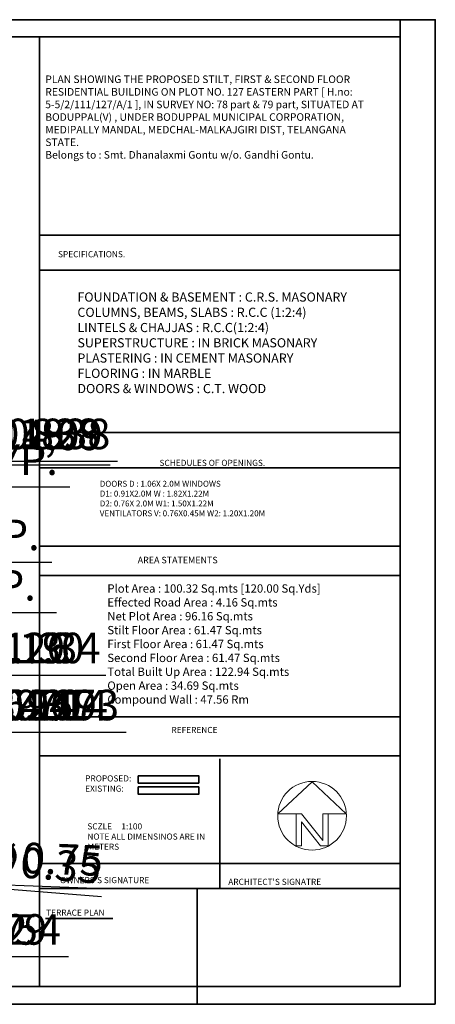
# Model space of a CAD drawing. Units: metres. Extents: x 782 to 1487, y 1262 to 7446.
# Tile 25 of 25: x 850 to 884, y 1262 to 1343. Entities that reach past the tile are written whole.
import ezdxf

# ---------------------------------------------------------------- set-up
doc = ezdxf.new("R2010")
doc.units = ezdxf.units.M
for name, color, linetype, lineweight in [('A-ANNO-DIMS', 2, 'Continuous', 18), ('A-ANNO-SYMB', 7, 'Continuous', 18), ('A-ANNO-TTLB', 7, 'Continuous', 35)]:
    doc.layers.add(name, color=color, linetype=linetype, lineweight=lineweight)
doc.styles.get("Standard").update_dxf_attribs({"font": 'arial.ttf'})
doc.dimstyles.new('ISO-25', dxfattribs={"dimtxt": 2.5, "dimasz": 2.5, "dimexe": 1.25, "dimexo": 0.625, "dimtad": 1, "dimtxsty": 'Standard', "dimcen": 2.5, "dimadec": 0, "dimazin": 0, "dimtfac": 1, "dimtmove": 0, "dimatfit": 3, "dimfxl": 1, "dimarcsym": 0})

# ---------------------------------------------------------------- blocks, each defined once
blk = doc.blocks.new('*D9')
at = {"layer": 'A-ANNO-DIMS', "color": 0, "lineweight": -2, "transparency": 16777216}
for p, q in [((840.095, 1306.46), (840.095, 1307.78)), ((844.185, 1306.46), (844.185, 1307.78)), ((837.595, 1306.53), (835.095, 1306.53)), ((840.095, 1306.53), (844.185, 1306.53)), ((846.685, 1306.53), (857.034, 1306.53))]:
    blk.add_line(p, q, dxfattribs=at)
at = {"layer": 'A-ANNO-DIMS', "color": 0, "transparency": 16777216}
for points in [[(837.595, 1306.947), (837.595, 1306.114), (840.095, 1306.53)], [(846.685, 1306.947), (846.685, 1306.114), (844.185, 1306.53)]]:
    blk.add_solid(points, dxfattribs=at)
at = {"layer": 'Defpoints', "color": 0, "transparency": 16777216}
for p in [(844.185, 1306.53), (840.095, 1305.835), (844.185, 1305.835)]:
    blk.add_point(p, dxfattribs=at)
at = {"layer": 'A-ANNO-DIMS', "color": 0, "transparency": 16777216, "insert": (853.11, 1308.658), "char_height": 2.5, "attachment_point": 5}
blk.add_mtext('4,09', dxfattribs=at)
blk = doc.blocks.new('North Arrow')
for p, q in [((0, 0), (-12.86, -11.999)), ((0, 0), (12.782, -11.999)), ((-12.86, -11.999), (-6, -11.999)), ((-6, -11.999), (-6, -23.999)), ((-6, -11.999), (-4, -11.999)), ((-4, -11.999), (4, -21.999)), ((4, -11.999), (4, -21.999)), ((6, -11.999), (4, -11.999)), ((12.782, -11.999), (6, -11.999)), ((6, -11.999), (6, -23.999)), ((3.195, -23.996), (-4, -15.002)), ((-4, -15.002), (-4, -23.999)), ((-6, -23.999), (-4, -23.999)), ((6, -23.999), (3.195, -23.999))]:
    blk.add_line(p, q)
blk.add_circle((-0.013, -12.745), 12.885)
blk = doc.blocks.new('*D21')
at = {"layer": 'A-ANNO-DIMS', "color": 0, "lineweight": -2, "transparency": 16777216}
for p, q in [((827.576, 1298.565), (825.076, 1298.565)), ((830.076, 1298.565), (830.923, 1298.565)), ((833.423, 1298.565), (852.255, 1298.565)), ((830.076, 1298.073), (830.076, 1297.315)), ((830.923, 1298.073), (830.923, 1297.315))]:
    blk.add_line(p, q, dxfattribs=at)
at = {"layer": 'A-ANNO-DIMS', "color": 0, "transparency": 16777216}
for points in [[(827.576, 1298.981), (827.576, 1298.148), (830.076, 1298.565)], [(833.423, 1298.981), (833.423, 1298.148), (830.923, 1298.565)]]:
    blk.add_solid(points, dxfattribs=at)
at = {"layer": 'Defpoints', "color": 0, "transparency": 16777216}
for p in [(830.076, 1298.698), (830.923, 1298.698), (830.923, 1298.565)]:
    blk.add_point(p, dxfattribs=at)
at = {"layer": 'A-ANNO-DIMS', "color": 0, "transparency": 16777216, "insert": (844.089, 1300.466), "char_height": 2.5, "attachment_point": 5}
blk.add_mtext('0.85 TYP.', dxfattribs=at)
blk = doc.blocks.new('*D24')
at = {"layer": 'A-ANNO-DIMS', "color": 0, "lineweight": -2, "transparency": 16777216}
for p, q in [((811.209, 1294.423), (808.709, 1294.423)), ((813.709, 1294.423), (814.559, 1294.423)), ((817.059, 1294.423), (852.649, 1294.423)), ((813.709, 1293.926), (813.709, 1293.173)), ((814.559, 1293.926), (814.559, 1293.173))]:
    blk.add_line(p, q, dxfattribs=at)
at = {"layer": 'A-ANNO-DIMS', "color": 0, "transparency": 16777216}
for points in [[(811.209, 1294.84), (811.209, 1294.006), (813.709, 1294.423)], [(817.059, 1294.84), (817.059, 1294.006), (814.559, 1294.423)]]:
    blk.add_solid(points, dxfattribs=at)
at = {"layer": 'Defpoints', "color": 0, "transparency": 16777216}
for p in [(813.709, 1294.551), (814.559, 1294.551), (814.559, 1294.423)]:
    blk.add_point(p, dxfattribs=at)
at = {"layer": 'A-ANNO-DIMS', "color": 0, "transparency": 16777216, "insert": (836.104, 1296.342), "char_height": 2.5, "attachment_point": 5}
blk.add_mtext('DOOR D2 0.85 TYP.', dxfattribs=at)
blk = doc.blocks.new('*D29')
at = {"layer": 'A-ANNO-DIMS', "color": 0, "lineweight": -2, "transparency": 16777216}
for p, q in [((829.683, 1304.73), (827.183, 1304.73)), ((832.183, 1304.73), (832.413, 1304.73)), ((832.183, 1304.242), (832.183, 1303.48)), ((832.413, 1304.242), (832.413, 1303.48)), ((834.913, 1304.73), (853.745, 1304.73))]:
    blk.add_line(p, q, dxfattribs=at)
at = {"layer": 'A-ANNO-DIMS', "color": 0, "transparency": 16777216}
for points in [[(829.683, 1305.146), (829.683, 1304.313), (832.183, 1304.73)], [(834.913, 1305.146), (834.913, 1304.313), (832.413, 1304.73)]]:
    blk.add_solid(points, dxfattribs=at)
at = {"layer": 'Defpoints', "color": 0, "transparency": 16777216}
for p in [(832.183, 1304.867), (832.413, 1304.867), (832.413, 1304.73)]:
    blk.add_point(p, dxfattribs=at)
at = {"layer": 'A-ANNO-DIMS', "color": 0, "transparency": 16777216, "insert": (845.579, 1306.632), "char_height": 2.5, "attachment_point": 5}
blk.add_mtext('0.23 TYP.', dxfattribs=at)
blk = doc.blocks.new('*D101')
at = {"layer": 'A-ANNO-DIMS', "color": 0, "lineweight": -2, "transparency": 16777216}
for p, q in [((840.091, 1306.46), (840.091, 1308.085)), ((841.28, 1306.46), (841.28, 1308.085)), ((837.591, 1306.835), (835.091, 1306.835)), ((840.091, 1306.835), (841.28, 1306.835)), ((843.78, 1306.835), (853.794, 1306.835))]:
    blk.add_line(p, q, dxfattribs=at)
at = {"layer": 'A-ANNO-DIMS', "color": 0, "transparency": 16777216}
for points in [[(837.591, 1307.252), (837.591, 1306.419), (840.091, 1306.835)], [(843.78, 1307.252), (843.78, 1306.419), (841.28, 1306.835)]]:
    blk.add_solid(points, dxfattribs=at)
at = {"layer": 'Defpoints', "color": 0, "transparency": 16777216}
for p in [(841.28, 1306.835), (840.091, 1305.835), (841.28, 1305.835)]:
    blk.add_point(p, dxfattribs=at)
at = {"layer": 'A-ANNO-DIMS', "color": 0, "transparency": 16777216, "insert": (850.037, 1308.737), "char_height": 2.5, "attachment_point": 5}
blk.add_mtext('1.19', dxfattribs=at)
blk = doc.blocks.new('*D102')
at = {"layer": 'A-ANNO-DIMS', "color": 0, "lineweight": -2, "transparency": 16777216}
for p, q in [((841.28, 1306.46), (841.28, 1308.085)), ((842.118, 1306.46), (842.118, 1308.085)), ((838.78, 1306.835), (836.28, 1306.835)), ((841.28, 1306.835), (842.118, 1306.835)), ((844.618, 1306.835), (856.81, 1306.835))]:
    blk.add_line(p, q, dxfattribs=at)
at = {"layer": 'A-ANNO-DIMS', "color": 0, "transparency": 16777216}
for points in [[(838.78, 1307.252), (838.78, 1306.419), (841.28, 1306.835)], [(844.618, 1307.252), (844.618, 1306.419), (842.118, 1306.835)]]:
    blk.add_solid(points, dxfattribs=at)
at = {"layer": 'Defpoints', "color": 0, "transparency": 16777216}
for p in [(842.118, 1306.835), (841.28, 1305.835), (842.118, 1305.835)]:
    blk.add_point(p, dxfattribs=at)
at = {"layer": 'A-ANNO-DIMS', "color": 0, "transparency": 16777216, "insert": (851.964, 1308.738), "char_height": 2.5, "attachment_point": 5}
blk.add_mtext('0.838', dxfattribs=at)
blk = doc.blocks.new('*D103')
at = {"layer": 'A-ANNO-DIMS', "color": 0, "lineweight": -2, "transparency": 16777216}
for p, q in [((842.118, 1306.46), (842.118, 1308.085)), ((842.956, 1306.46), (842.956, 1308.085)), ((839.618, 1306.835), (837.118, 1306.835)), ((842.118, 1306.835), (842.956, 1306.835)), ((845.456, 1306.835), (857.648, 1306.835))]:
    blk.add_line(p, q, dxfattribs=at)
at = {"layer": 'A-ANNO-DIMS', "color": 0, "transparency": 16777216}
for points in [[(839.618, 1307.252), (839.618, 1306.419), (842.118, 1306.835)], [(845.456, 1307.252), (845.456, 1306.419), (842.956, 1306.835)]]:
    blk.add_solid(points, dxfattribs=at)
at = {"layer": 'Defpoints', "color": 0, "transparency": 16777216}
for p in [(842.956, 1306.835), (842.118, 1305.835), (842.956, 1305.835)]:
    blk.add_point(p, dxfattribs=at)
at = {"layer": 'A-ANNO-DIMS', "color": 0, "transparency": 16777216, "insert": (852.802, 1308.738), "char_height": 2.5, "attachment_point": 5}
blk.add_mtext('0.838', dxfattribs=at)
blk = doc.blocks.new('*D104')
at = {"layer": 'A-ANNO-DIMS', "color": 0, "lineweight": -2, "transparency": 16777216}
for p, q in [((842.956, 1306.46), (842.956, 1308.085)), ((844.185, 1306.46), (844.185, 1308.085)), ((840.456, 1306.835), (837.956, 1306.835)), ((842.956, 1306.835), (844.185, 1306.835)), ((846.685, 1306.835), (856.693, 1306.835))]:
    blk.add_line(p, q, dxfattribs=at)
at = {"layer": 'A-ANNO-DIMS', "color": 0, "transparency": 16777216}
for points in [[(840.456, 1307.252), (840.456, 1306.419), (842.956, 1306.835)], [(846.685, 1307.252), (846.685, 1306.419), (844.185, 1306.835)]]:
    blk.add_solid(points, dxfattribs=at)
at = {"layer": 'Defpoints', "color": 0, "transparency": 16777216}
for p in [(844.185, 1306.835), (842.956, 1305.835), (844.185, 1305.835)]:
    blk.add_point(p, dxfattribs=at)
at = {"layer": 'A-ANNO-DIMS', "color": 0, "transparency": 16777216, "insert": (852.939, 1308.738), "char_height": 2.5, "attachment_point": 5}
blk.add_mtext('1.23', dxfattribs=at)
blk = doc.blocks.new('*D105')
at = {"layer": 'A-ANNO-DIMS', "color": 0, "lineweight": -2, "transparency": 16777216}
for p, q in [((840.091, 1289.68), (840.091, 1288.055)), ((841.28, 1289.68), (841.28, 1288.055)), ((837.591, 1289.305), (835.091, 1289.305)), ((840.091, 1289.305), (841.28, 1289.305)), ((843.78, 1289.305), (853.794, 1289.305))]:
    blk.add_line(p, q, dxfattribs=at)
at = {"layer": 'A-ANNO-DIMS', "color": 0, "transparency": 16777216}
for points in [[(837.591, 1289.722), (837.591, 1288.889), (840.091, 1289.305)], [(843.78, 1289.722), (843.78, 1288.889), (841.28, 1289.305)]]:
    blk.add_solid(points, dxfattribs=at)
at = {"layer": 'Defpoints', "color": 0, "transparency": 16777216}
for p in [(840.091, 1290.305), (841.28, 1290.305), (841.28, 1289.305)]:
    blk.add_point(p, dxfattribs=at)
at = {"layer": 'A-ANNO-DIMS', "color": 0, "transparency": 16777216, "insert": (850.037, 1291.207), "char_height": 2.5, "attachment_point": 5}
blk.add_mtext('1.19', dxfattribs=at)
blk = doc.blocks.new('*D106')
at = {"layer": 'A-ANNO-DIMS', "color": 0, "lineweight": -2, "transparency": 16777216}
for p, q in [((841.28, 1289.68), (841.28, 1288.055)), ((841.541, 1289.68), (841.541, 1288.055)), ((838.78, 1289.305), (836.28, 1289.305)), ((841.28, 1289.305), (841.541, 1289.305)), ((844.041, 1289.305), (854.283, 1289.305))]:
    blk.add_line(p, q, dxfattribs=at)
at = {"layer": 'A-ANNO-DIMS', "color": 0, "transparency": 16777216}
for points in [[(838.78, 1289.722), (838.78, 1288.889), (841.28, 1289.305)], [(844.041, 1289.722), (844.041, 1288.889), (841.541, 1289.305)]]:
    blk.add_solid(points, dxfattribs=at)
at = {"layer": 'Defpoints', "color": 0, "transparency": 16777216}
for p in [(841.28, 1290.305), (841.541, 1290.305), (841.541, 1289.305)]:
    blk.add_point(p, dxfattribs=at)
at = {"layer": 'A-ANNO-DIMS', "color": 0, "transparency": 16777216, "insert": (850.412, 1291.207), "char_height": 2.5, "attachment_point": 5}
blk.add_mtext('0.26', dxfattribs=at)
blk = doc.blocks.new('*D107')
at = {"layer": 'A-ANNO-DIMS', "color": 0, "lineweight": -2, "transparency": 16777216}
for p, q in [((841.541, 1289.68), (841.541, 1288.055)), ((842.844, 1289.68), (842.844, 1288.055)), ((839.041, 1289.305), (836.541, 1289.305)), ((841.541, 1289.305), (842.844, 1289.305)), ((845.344, 1289.305), (855.344, 1289.305))]:
    blk.add_line(p, q, dxfattribs=at)
at = {"layer": 'A-ANNO-DIMS', "color": 0, "transparency": 16777216}
for points in [[(839.041, 1289.722), (839.041, 1288.889), (841.541, 1289.305)], [(845.344, 1289.722), (845.344, 1288.889), (842.844, 1289.305)]]:
    blk.add_solid(points, dxfattribs=at)
at = {"layer": 'Defpoints', "color": 0, "transparency": 16777216}
for p in [(841.541, 1290.305), (842.844, 1290.305), (842.844, 1289.305)]:
    blk.add_point(p, dxfattribs=at)
at = {"layer": 'A-ANNO-DIMS', "color": 0, "transparency": 16777216, "insert": (851.594, 1291.208), "char_height": 2.5, "attachment_point": 5}
blk.add_mtext('1.30', dxfattribs=at)
blk = doc.blocks.new('*D108')
at = {"layer": 'A-ANNO-DIMS', "color": 0, "lineweight": -2, "transparency": 16777216}
for p, q in [((842.844, 1289.68), (842.844, 1288.055)), ((844.185, 1289.68), (844.185, 1288.055)), ((840.344, 1289.305), (837.844, 1289.305)), ((842.844, 1289.305), (844.185, 1289.305)), ((846.685, 1289.305), (856.683, 1289.305))]:
    blk.add_line(p, q, dxfattribs=at)
at = {"layer": 'A-ANNO-DIMS', "color": 0, "transparency": 16777216}
for points in [[(840.344, 1289.722), (840.344, 1288.889), (842.844, 1289.305)], [(846.685, 1289.722), (846.685, 1288.889), (844.185, 1289.305)]]:
    blk.add_solid(points, dxfattribs=at)
at = {"layer": 'Defpoints', "color": 0, "transparency": 16777216}
for p in [(842.844, 1290.305), (844.185, 1290.305), (844.185, 1289.305)]:
    blk.add_point(p, dxfattribs=at)
at = {"layer": 'A-ANNO-DIMS', "color": 0, "transparency": 16777216, "insert": (852.934, 1291.208), "char_height": 2.5, "attachment_point": 5}
blk.add_mtext('1.34', dxfattribs=at)
blk = doc.blocks.new('*D149')
at = {"layer": 'A-ANNO-DIMS', "color": 0, "lineweight": -2, "transparency": 16777216}
for p, q in [((836.744, 1268.517), (836.744, 1265.001)), ((838.898, 1268.517), (838.898, 1265.001)), ((834.244, 1266.251), (831.744, 1266.251)), ((836.744, 1266.251), (838.898, 1266.251)), ((841.398, 1266.251), (853.616, 1266.251))]:
    blk.add_line(p, q, dxfattribs=at)
at = {"layer": 'A-ANNO-DIMS', "color": 0, "transparency": 16777216}
for points in [[(834.244, 1266.668), (834.244, 1265.835), (836.744, 1266.251)], [(841.398, 1266.668), (841.398, 1265.835), (838.898, 1266.251)]]:
    blk.add_solid(points, dxfattribs=at)
at = {"layer": 'Defpoints', "color": 0, "transparency": 16777216}
for p in [(836.744, 1269.142), (838.898, 1269.142), (838.898, 1266.251)]:
    blk.add_point(p, dxfattribs=at)
at = {"layer": 'A-ANNO-DIMS', "color": 0, "transparency": 16777216, "insert": (848.757, 1268.153), "char_height": 2.5, "attachment_point": 5}
blk.add_mtext('2.154', dxfattribs=at)
blk = doc.blocks.new('*D150')
at = {"layer": 'A-ANNO-DIMS', "color": 0, "lineweight": -2, "transparency": 16777216}
for p, q in [((838.898, 1268.517), (838.898, 1265.001)), ((839.686, 1268.517), (839.686, 1265.001)), ((836.398, 1266.251), (833.898, 1266.251)), ((838.898, 1266.251), (839.686, 1266.251)), ((842.186, 1266.251), (852.435, 1266.251))]:
    blk.add_line(p, q, dxfattribs=at)
at = {"layer": 'A-ANNO-DIMS', "color": 0, "transparency": 16777216}
for points in [[(836.398, 1266.668), (836.398, 1265.835), (838.898, 1266.251)], [(842.186, 1266.668), (842.186, 1265.835), (839.686, 1266.251)]]:
    blk.add_solid(points, dxfattribs=at)
at = {"layer": 'Defpoints', "color": 0, "transparency": 16777216}
for p in [(838.898, 1269.142), (839.686, 1269.142), (839.686, 1266.251)]:
    blk.add_point(p, dxfattribs=at)
at = {"layer": 'A-ANNO-DIMS', "color": 0, "transparency": 16777216, "insert": (848.561, 1268.153), "char_height": 2.5, "attachment_point": 5}
blk.add_mtext('0.79', dxfattribs=at)
blk = doc.blocks.new('*D151')
at = {"layer": 'A-ANNO-DIMS', "color": 0, "lineweight": -2, "transparency": 16777216}
for p, q in [((839.686, 1273.694), (839.686, 1285.879)), ((841.835, 1273.694), (841.835, 1285.879)), ((837.186, 1284.629), (834.686, 1284.629)), ((839.686, 1284.629), (841.835, 1284.629)), ((844.335, 1284.629), (856.569, 1284.629))]:
    blk.add_line(p, q, dxfattribs=at)
at = {"layer": 'A-ANNO-DIMS', "color": 0, "transparency": 16777216}
for points in [[(837.186, 1285.046), (837.186, 1284.212), (839.686, 1284.629)], [(844.335, 1285.046), (844.335, 1284.212), (841.835, 1284.629)]]:
    blk.add_solid(points, dxfattribs=at)
at = {"layer": 'Defpoints', "color": 0, "transparency": 16777216}
for p in [(841.835, 1284.629), (839.686, 1273.069), (841.835, 1273.069)]:
    blk.add_point(p, dxfattribs=at)
at = {"layer": 'A-ANNO-DIMS', "color": 0, "transparency": 16777216, "insert": (851.702, 1286.531), "char_height": 2.5, "attachment_point": 5}
blk.add_mtext('2.149', dxfattribs=at)
blk = doc.blocks.new('*D152')
at = {"layer": 'A-ANNO-DIMS', "color": 0, "lineweight": -2, "transparency": 16777216}
for p, q in [((841.835, 1273.694), (841.835, 1285.879)), ((842.533, 1273.678), (842.533, 1285.879)), ((839.335, 1284.629), (836.835, 1284.629)), ((841.835, 1284.629), (842.533, 1284.629)), ((845.033, 1284.629), (855.269, 1284.629))]:
    blk.add_line(p, q, dxfattribs=at)
at = {"layer": 'A-ANNO-DIMS', "color": 0, "transparency": 16777216}
for points in [[(839.335, 1285.046), (839.335, 1284.212), (841.835, 1284.629)], [(845.033, 1285.046), (845.033, 1284.212), (842.533, 1284.629)]]:
    blk.add_solid(points, dxfattribs=at)
at = {"layer": 'Defpoints', "color": 0, "transparency": 16777216}
for p in [(842.533, 1284.629), (841.835, 1273.069), (842.533, 1273.053)]:
    blk.add_point(p, dxfattribs=at)
at = {"layer": 'A-ANNO-DIMS', "color": 0, "transparency": 16777216, "insert": (851.401, 1286.531), "char_height": 2.5, "attachment_point": 5}
blk.add_mtext('0.70', dxfattribs=at)
blk = doc.blocks.new('*D153')
at = {"layer": 'A-ANNO-DIMS', "color": 0, "lineweight": -2, "transparency": 16777216}
for p, q in [((842.533, 1273.678), (842.533, 1285.879)), ((844.669, 1273.698), (844.669, 1285.879)), ((840.033, 1284.629), (837.533, 1284.629)), ((842.533, 1284.629), (844.669, 1284.629)), ((847.169, 1284.629), (857.445, 1284.629))]:
    blk.add_line(p, q, dxfattribs=at)
at = {"layer": 'A-ANNO-DIMS', "color": 0, "transparency": 16777216}
for points in [[(840.033, 1285.046), (840.033, 1284.212), (842.533, 1284.629)], [(847.169, 1285.046), (847.169, 1284.212), (844.669, 1284.629)]]:
    blk.add_solid(points, dxfattribs=at)
at = {"layer": 'Defpoints', "color": 0, "transparency": 16777216}
for p in [(844.669, 1284.629), (842.533, 1273.053), (844.669, 1273.073)]:
    blk.add_point(p, dxfattribs=at)
at = {"layer": 'A-ANNO-DIMS', "color": 0, "transparency": 16777216, "insert": (853.557, 1286.509), "char_height": 2.5, "attachment_point": 5}
blk.add_mtext('2.14', dxfattribs=at)
blk = doc.blocks.new('*D155')
at = {"layer": 'A-ANNO-DIMS', "color": 0, "lineweight": -2, "transparency": 16777216}
for p, q in [((837.496, 1270.243), (837.496, 1265.001)), ((838.116, 1270.243), (838.116, 1265.001)), ((834.996, 1266.251), (832.496, 1266.251)), ((837.496, 1266.251), (838.116, 1266.251)), ((840.616, 1266.251), (850.834, 1266.251))]:
    blk.add_line(p, q, dxfattribs=at)
at = {"layer": 'A-ANNO-DIMS', "color": 0, "transparency": 16777216}
for points in [[(834.996, 1266.668), (834.996, 1265.835), (837.496, 1266.251)], [(840.616, 1266.668), (840.616, 1265.835), (838.116, 1266.251)]]:
    blk.add_solid(points, dxfattribs=at)
at = {"layer": 'Defpoints', "color": 0, "transparency": 16777216}
for p in [(837.496, 1270.868), (838.116, 1270.868), (838.116, 1266.251)]:
    blk.add_point(p, dxfattribs=at)
at = {"layer": 'A-ANNO-DIMS', "color": 0, "transparency": 16777216, "insert": (846.975, 1268.153), "char_height": 2.5, "attachment_point": 5}
blk.add_mtext('0.62', dxfattribs=at)
blk = doc.blocks.new('*D156')
at = {"layer": 'A-ANNO-DIMS', "color": 0, "lineweight": -2, "transparency": 16777216}
for p, q in [((836.503, 1283.244), (836.503, 1285.879)), ((846.176, 1283.244), (846.176, 1285.879)), ((839.003, 1284.629), (843.676, 1284.629)), ((846.176, 1284.629), (858.362, 1284.629))]:
    blk.add_line(p, q, dxfattribs=at)
at = {"layer": 'A-ANNO-DIMS', "color": 0, "transparency": 16777216}
for points in [[(839.003, 1285.046), (839.003, 1284.212), (836.503, 1284.629)], [(843.676, 1285.046), (843.676, 1284.212), (846.176, 1284.629)]]:
    blk.add_solid(points, dxfattribs=at)
at = {"layer": 'Defpoints', "color": 0, "transparency": 16777216}
for p in [(846.176, 1284.629), (836.503, 1282.619), (846.176, 1282.619)]:
    blk.add_point(p, dxfattribs=at)
at = {"layer": 'A-ANNO-DIMS', "color": 0, "transparency": 16777216, "insert": (853.519, 1286.531), "char_height": 2.5, "attachment_point": 5}
blk.add_mtext('9.673', dxfattribs=at)
blk = doc.blocks.new('*D158')
at = {"layer": 'A-ANNO-DIMS', "color": 0, "lineweight": -2, "transparency": 16777216}
for p, q in [((836.503, 1283.244), (836.503, 1285.879)), ((837.132, 1282.644), (837.132, 1285.879)), ((834.003, 1284.629), (831.503, 1284.629)), ((836.503, 1284.629), (837.132, 1284.629)), ((839.632, 1284.629), (849.876, 1284.629))]:
    blk.add_line(p, q, dxfattribs=at)
at = {"layer": 'A-ANNO-DIMS', "color": 0, "transparency": 16777216}
for points in [[(834.003, 1285.046), (834.003, 1284.212), (836.503, 1284.629)], [(839.632, 1285.046), (839.632, 1284.212), (837.132, 1284.629)]]:
    blk.add_solid(points, dxfattribs=at)
at = {"layer": 'Defpoints', "color": 0, "transparency": 16777216}
for p in [(837.132, 1284.629), (836.503, 1282.619), (837.132, 1282.019)]:
    blk.add_point(p, dxfattribs=at)
at = {"layer": 'A-ANNO-DIMS', "color": 0, "transparency": 16777216, "insert": (846.004, 1286.531), "char_height": 2.5, "attachment_point": 5}
blk.add_mtext('0.63', dxfattribs=at)
blk = doc.blocks.new('*D159')
at = {"layer": 'A-ANNO-DIMS', "color": 0, "lineweight": -2, "transparency": 16777216}
for p, q in [((837.132, 1282.644), (837.132, 1285.879)), ((839.826, 1282.644), (839.826, 1285.879)), ((834.632, 1284.629), (832.132, 1284.629)), ((837.132, 1284.629), (839.826, 1284.629)), ((842.326, 1284.629), (854.545, 1284.629))]:
    blk.add_line(p, q, dxfattribs=at)
at = {"layer": 'A-ANNO-DIMS', "color": 0, "transparency": 16777216}
for points in [[(834.632, 1285.046), (834.632, 1284.212), (837.132, 1284.629)], [(842.326, 1285.046), (842.326, 1284.212), (839.826, 1284.629)]]:
    blk.add_solid(points, dxfattribs=at)
at = {"layer": 'Defpoints', "color": 0, "transparency": 16777216}
for p in [(839.826, 1284.629), (837.132, 1282.019), (839.826, 1282.019)]:
    blk.add_point(p, dxfattribs=at)
at = {"layer": 'A-ANNO-DIMS', "color": 0, "transparency": 16777216, "insert": (849.686, 1286.531), "char_height": 2.5, "attachment_point": 5}
blk.add_mtext('2.694', dxfattribs=at)
blk = doc.blocks.new('*D160')
at = {"layer": 'A-ANNO-DIMS', "color": 0, "lineweight": -2, "transparency": 16777216}
for p, q in [((839.826, 1280.313), (839.826, 1285.879)), ((841.255, 1280.444), (841.255, 1285.879)), ((837.326, 1284.629), (834.826, 1284.629)), ((839.826, 1284.629), (841.255, 1284.629)), ((843.755, 1284.629), (853.764, 1284.629))]:
    blk.add_line(p, q, dxfattribs=at)
at = {"layer": 'A-ANNO-DIMS', "color": 0, "transparency": 16777216}
for points in [[(837.326, 1285.046), (837.326, 1284.212), (839.826, 1284.629)], [(843.755, 1285.046), (843.755, 1284.212), (841.255, 1284.629)]]:
    blk.add_solid(points, dxfattribs=at)
at = {"layer": 'Defpoints', "color": 0, "transparency": 16777216}
for p in [(841.255, 1284.629), (841.255, 1279.819), (839.826, 1279.688)]:
    blk.add_point(p, dxfattribs=at)
at = {"layer": 'A-ANNO-DIMS', "color": 0, "transparency": 16777216, "insert": (850.01, 1286.531), "char_height": 2.5, "attachment_point": 5}
blk.add_mtext('1.43', dxfattribs=at)
blk = doc.blocks.new('*D171')
at = {"layer": 'A-ANNO-DIMS', "color": 0, "lineweight": -2, "transparency": 16777216}
for p, q in [((837.863, 1272.527), (835.364, 1272.625)), ((840.361, 1272.43), (841.106, 1272.401)), ((856.577, 1271.797), (843.604, 1272.303))]:
    blk.add_line(p, q, dxfattribs=at)
at = {"layer": 'A-ANNO-DIMS', "color": 0, "transparency": 16777216}
for points in [[(837.879, 1272.943), (837.846, 1272.111), (840.361, 1272.43)], [(843.621, 1272.719), (843.588, 1271.887), (841.106, 1272.401)]]:
    blk.add_solid(points, dxfattribs=at)
at = {"layer": 'Defpoints', "color": 0, "transparency": 16777216}
for p in [(840.361, 1272.43), (841.106, 1272.401)]:
    blk.add_point(p, dxfattribs=at)
at = {"layer": 'A-ANNO-DIMS', "color": 0, "transparency": 16777216, "insert": (851.417, 1273.971), "char_height": 2.5, "attachment_point": 5, "rotation": 357.76587}
blk.add_mtext('∅0.75', dxfattribs=at)
blk = doc.blocks.new('*D172')
at = {"layer": 'A-ANNO-DIMS', "color": 0, "lineweight": -2, "transparency": 16777216}
for p, q in [((838.066, 1272.631), (835.574, 1272.832)), ((840.558, 1272.429), (840.909, 1272.401)), ((856.341, 1271.153), (843.401, 1272.199))]:
    blk.add_line(p, q, dxfattribs=at)
at = {"layer": 'A-ANNO-DIMS', "color": 0, "transparency": 16777216}
for points in [[(838.1, 1273.046), (838.032, 1272.215), (840.558, 1272.429)], [(843.435, 1272.615), (843.367, 1271.784), (840.909, 1272.401)]]:
    blk.add_solid(points, dxfattribs=at)
at = {"layer": 'Defpoints', "color": 0, "transparency": 16777216}
for p in [(840.558, 1272.429), (840.909, 1272.401)]:
    blk.add_point(p, dxfattribs=at)
at = {"layer": 'A-ANNO-DIMS', "color": 0, "transparency": 16777216, "insert": (851.276, 1273.541), "char_height": 2.5, "attachment_point": 5, "rotation": 355.37805}
blk.add_mtext('∅0.35', dxfattribs=at)

msp = doc.modelspace()

# ---------------------------------------------------------------- linework, layer by layer
at = {"layer": 'A-ANNO-TTLB'}
for p, q in [((834.8075, 1341.5907), (851.2547, 1341.5907)), ((851.2547, 1341.5907), (851.2547, 1263.8004)), ((851.2547, 1341.5907), (851.2547, 1322.4835)), ((851.2547, 1325.3258), (880.8003, 1325.3258)), ((851.2547, 1322.4835), (880.8003, 1322.4835)), ((880.8003, 1322.4835), (880.8003, 1306.2827)), ((880.8003, 1309.1816), (851.2547, 1309.1816)), ((880.8003, 1306.2827), (851.2547, 1306.2827)), ((851.2547, 1306.2827), (851.2547, 1297.4622)), ((851.2547, 1299.8543), (880.8003, 1299.8543)), ((851.2547, 1297.4622), (880.8003, 1297.4622)), ((880.8003, 1297.4622), (880.8003, 1281.0813)), ((880.8003, 1285.8966), (851.2547, 1285.8966)), ((880.8003, 1282.6906), (851.2547, 1282.6906)), ((866.0275, 1282.4636), (866.0275, 1271.8196)), ((851.2547, 1281.0813), (851.2547, 1273.881)), ((851.2547, 1273.881), (880.8003, 1273.881)), ((851.2547, 1271.8196), (880.8003, 1271.8196)), ((866.0275, 1271.8196), (864.1769, 1271.8196)), ((864.1769, 1271.8196), (864.1769, 1262.3458)), ((851.7556, 1269.3814), (857.2501, 1269.3814))]:
    msp.add_line(p, q, dxfattribs=at)
for points in [[(787.4248, 1342.9861), (880.8003, 1342.9861), (880.8003, 1263.8004), (787.4248, 1263.8004)], [(883.6865, 1262.3458), (787.4248, 1262.3458), (787.4248, 1342.9861), (883.6865, 1342.9861)], [(788.8147, 1341.5907), (880.8003, 1341.5907), (880.8003, 1263.8004), (788.8147, 1263.8004)], [(859.3481, 1281.0614), (864.2985, 1281.0614), (864.2985, 1280.4619), (859.3481, 1280.4619)], [(859.3481, 1280.1436), (864.2985, 1280.1436), (864.2985, 1279.5441), (859.3481, 1279.5441)]]:
    msp.add_lwpolyline(points, close=True, dxfattribs=at)

# ---------------------------------------------------------------- block references
at = {"layer": 'A-ANNO-SYMB', "xscale": 0.2183538714177247, "yscale": 0.2183538714177247, "zscale": 0.2183538714177247}
msp.add_blockref('North Arrow', (873.5926, 1280.5661), dxfattribs=at)

# ---------------------------------------------------------------- texts
at = {"layer": 'A-ANNO-TTLB', "attachment_point": 1}
for s, insert, char_height, width in [('PLAN SHOWING THE PROPOSED STILT, FIRST & SECOND FLOOR\\PRESIDENTIAL BUILDING ON PLOT NO. 127 EASTERN PART [ H.no:\\P5-5/2/111/127/A/1 ], IN SURVEY NO: 78 part & 79 part, SITUATED AT\\PBODUPPAL(V) , UNDER BODUPPAL MUNICIPAL CORPORATION,\\PMEDIPALLY MANDAL, MEDCHAL-MALKAJGIRI DIST, TELANGANA\\PSTATE.\\P Belongs to : Smt. Dhanalaxmi Gontu w/o. Gandhi Gontu.', (851.7248, 1338.4173), 0.619071, 28.678234), ('FOUNDATION & BASEMENT : C.R.S. MASONARY\\PCOLUMNS, BEAMS, SLABS : R.C.C (1:2:4)\\PLINTELS & CHAJJAS : R.C.C(1:2:4)\\PSUPERSTRUCTURE : IN BRICK MASONARY\\PPLASTERING : IN CEMENT MASONARY\\PFLOORING : IN MARBLE\\PDOORS & WINDOWS : C.T. WOOD', (854.3587, 1320.6471), 0.749576, 25.315146), ('DOORS D : 1.06X 2.0M WINDOWS\\P D1: 0.91X2.0M W : 1.82X1.22M\\P D2: 0.76X 2.0M W1: 1.50X1.22M\\PVENTILATORS V: 0.76X0.45M W2: 1.20X1.20M', (856.1886, 1305.2225), 0.484681, 15.274749), ('Plot Area : 100.32 Sq.mts [120.00 Sq.Yds]\\PEffected Road Area : 4.16 Sq.mts\\PNet Plot Area : 96.16 Sq.mts\\PStilt Floor Area : 61.47 Sq.mts\\PFirst Floor Area : 61.47 Sq.mts\\PSecond Floor Area : 61.47 Sq.mts\\PTotal Built Up Area : 122.94 Sq.mts\\POpen Area : 34.69 Sq.mts\\PCompound Wall : 47.56 Rm', (856.8086, 1296.7425), 0.681833, 18.649686)]:
    msp.add_mtext(s, dxfattribs=dict(at, insert=insert, char_height=char_height, width=width))
for s, width, gutter_width, heights, insert, char_height in [('\\PSPECIFICATIONS.', 17.304543, 12.5, [0], (852.7684, 1324.8642), 0.5), ('\\PSCHEDULES OF OPENINGS. ', 12.064323, 6.2373, [0], (861.0824, 1307.7749), 0.5), ('AREA STATEMENTS', 21.700943, 23.3313, [0.9199], (859.2983, 1298.9986), 0.535314), ('\\PREFERENCE', 15.426673, 12.5, [0], (862.0617, 1285.8966), 0.5), ('\\PPROPOSED:\\PEXISTING:', 20.791463, 12.5, [0], (854.9938, 1281.9287), 0.5), ('\\PSCZLE     1:100\\PNOTE ALL DIMENSINOS ARE IN METERS', 10.857944, 12.5, [0], (855.1696, 1278.0013), 0.5), ("\\POWNERS'S SIGNATURE", 8.083861, 12.5, [0], (852.9369, 1273.6006), 0.5), ("\\PARCHITECT'S SIGNATRE", 10.607573, 12.5, [0], (866.7189, 1273.4613), 0.5), ('\\PTERRACE PLAN', 10.508783, 12.5, [0], (851.794, 1270.9363), 0.5)]:
    msp.add_mtext_dynamic_manual_height_columns(s, width=width, gutter_width=gutter_width, heights=heights, dxfattribs=dict(at, insert=insert, char_height=char_height))

# ---------------------------------------------------------------- dimensions: what is measured, and where the dimension line sits
at = {"layer": 'A-ANNO-DIMS'}
for base, p1, p2, text, picture, middle in [((832.4132, 1304.7298), (832.1832, 1304.8669), (832.4132, 1304.8669), '<> TYP.', '*D29', (845.5791, 1306.6321)), ((814.5592, 1294.4231), (813.7086, 1294.5507), (814.5592, 1294.5507), 'DOOR D2 <> TYP.', '*D24', (836.1042, 1296.3416)), ((830.923, 1298.5648), (830.0763, 1298.6982), (830.923, 1298.6982), '<> TYP.', '*D21', (844.0889, 1300.4662))]:
    dim = msp.add_linear_dim(base=base, p1=p1, p2=p2, text=text, dimstyle='ISO-25', override={"dimdec": 2, "dimlfac": 1, "dimrnd": 0, "dimzin": 0, "dimdsep": 46, "dimlunit": 2}, dxfattribs=at)
    dim.commit()
    dim.dimension.update_dxf_attribs({"geometry": picture, "text_midpoint": middle})
for base, p1, p2, override, picture, middle in [((841.2801, 1306.8353), (840.0913, 1305.8353), (841.2801, 1305.8353), {"dimdec": 2, "dimlfac": 1, "dimrnd": 0, "dimzin": 0, "dimdsep": 46, "dimlunit": 2}, '*D101', (850.037, 1308.7367)), ((844.1849, 1306.5303), (840.0949, 1305.8353), (844.1849, 1305.8353), {"dimclrd": 0, "dimclre": 0, "dimclrt": 0}, '*D9', (853.1097, 1308.6577)), ((842.1182, 1306.8353), (841.2801, 1305.8353), (842.1182, 1305.8353), {"dimdec": 3, "dimlfac": 1, "dimrnd": 0, "dimzin": 0, "dimdsep": 46, "dimlunit": 2}, '*D102', (851.9639, 1308.7376)), ((842.9563, 1306.8353), (842.1182, 1305.8353), (842.9563, 1305.8353), {"dimdec": 3, "dimlfac": 1, "dimrnd": 0, "dimzin": 0, "dimdsep": 46, "dimlunit": 2}, '*D103', (852.802, 1308.7376)), ((844.1849, 1306.8353), (842.9563, 1305.8353), (844.1849, 1305.8353), {"dimdec": 2, "dimlfac": 1, "dimrnd": 0, "dimzin": 0, "dimdsep": 46, "dimlunit": 2}, '*D104', (852.9391, 1308.7376)), ((841.2801, 1289.3053), (840.0913, 1290.3053), (841.2801, 1290.3053), {"dimdec": 2, "dimlfac": 1, "dimrnd": 0, "dimzin": 0, "dimdsep": 46, "dimlunit": 2}, '*D105', (850.037, 1291.2067)), ((841.5409, 1289.3053), (841.2801, 1290.3053), (841.5409, 1290.3053), {"dimdec": 2, "dimlfac": 1, "dimrnd": 0, "dimzin": 0, "dimdsep": 46, "dimlunit": 2}, '*D106', (850.4119, 1291.2067)), ((842.8445, 1289.3053), (841.5409, 1290.3053), (842.8445, 1290.3053), {"dimdec": 2, "dimlfac": 1, "dimrnd": 0, "dimzin": 0, "dimdsep": 46, "dimlunit": 2}, '*D107', (851.5945, 1291.2076)), ((844.1849, 1289.3053), (842.8445, 1290.3053), (844.1849, 1290.3053), {"dimdec": 2, "dimlfac": 1, "dimrnd": 0, "dimzin": 0, "dimdsep": 46, "dimlunit": 2}, '*D108', (852.934, 1291.2076)), ((837.1321, 1284.6291), (836.5033, 1282.619), (837.1321, 1282.0186), {"dimdec": 2, "dimlfac": 1, "dimrnd": 0, "dimzin": 0, "dimdsep": 46, "dimlunit": 2}, '*D158', (846.004, 1286.5314)), ((839.8262, 1284.6291), (837.1321, 1282.0186), (839.8262, 1282.0186), {"dimdec": 3, "dimlfac": 1, "dimrnd": 0, "dimzin": 0, "dimdsep": 46, "dimlunit": 2}, '*D159', (849.6855, 1286.5306)), ((841.835, 1284.6291), (839.686, 1273.0692), (841.835, 1273.0692), {"dimdec": 3, "dimlfac": 1, "dimrnd": 0, "dimzin": 0, "dimdsep": 46, "dimlunit": 2}, '*D151', (851.702, 1286.5306)), ((841.2554, 1284.6291), (839.8262, 1279.6878), (841.2554, 1279.8192), {"dimdec": 2, "dimlfac": 1, "dimrnd": 0, "dimzin": 0, "dimdsep": 46, "dimlunit": 2}, '*D160', (850.0097, 1286.5314)), ((846.1759, 1284.6291), (836.5033, 1282.619), (846.1759, 1282.619), {"dimdec": 3, "dimlfac": 1, "dimrnd": 0, "dimzin": 0, "dimdsep": 46, "dimlunit": 2}, '*D156', (853.519, 1286.5314)), ((842.5333, 1284.6291), (841.835, 1273.0692), (842.5333, 1273.0533), {"dimdec": 2, "dimlfac": 1, "dimrnd": 0, "dimzin": 0, "dimdsep": 46, "dimlunit": 2}, '*D152', (851.4009, 1286.5306)), ((844.6687, 1284.6291), (842.5333, 1273.0533), (844.6687, 1273.0726), {"dimdec": 2, "dimlfac": 1, "dimrnd": 0, "dimzin": 0, "dimdsep": 46, "dimlunit": 2}, '*D153', (853.5568, 1286.5093)), ((838.1156, 1266.2514), (837.496, 1270.8681), (838.1156, 1270.8681), {"dimdec": 2, "dimlfac": 1, "dimrnd": 0, "dimzin": 0, "dimdsep": 46, "dimlunit": 2}, '*D155', (846.9747, 1268.1528)), ((838.8977, 1266.2514), (836.7437, 1269.1422), (838.8977, 1269.1422), {"dimdec": 3, "dimlfac": 1, "dimrnd": 0, "dimzin": 0, "dimdsep": 46, "dimlunit": 2}, '*D149', (848.757, 1268.1528)), ((839.686, 1266.2514), (838.8977, 1269.1422), (839.686, 1269.1422), {"dimdec": 2, "dimlfac": 1, "dimrnd": 0, "dimzin": 0, "dimdsep": 46, "dimlunit": 2}, '*D150', (848.5605, 1268.1528))]:
    dim = msp.add_linear_dim(base=base, p1=p1, p2=p2, dimstyle='ISO-25', override=override, dxfattribs=at)
    dim.commit()
    dim.dimension.update_dxf_attribs({"geometry": picture, "text_midpoint": middle})
dim = msp.add_diameter_dim_2p(p1=(840.3606, 1272.4296), p2=(841.1063, 1272.4005), dimstyle='ISO-25', override={"dimdec": 2, "dimlfac": 1, "dimrnd": 0, "dimzin": 0, "dimdsep": 46, "dimlunit": 2}, dxfattribs=at)
dim.commit()
dim.dimension.update_dxf_attribs({"geometry": '*D171', "text_midpoint": (851.3398, 1272.0013)})
dim = msp.add_diameter_dim_2p(p1=(840.5578, 1272.4293), p2=(840.9091, 1272.4009), dimstyle='ISO-25', override={"dimdec": 2, "dimlfac": 1, "dimrnd": 0, "dimzin": 0, "dimdsep": 46, "dimlunit": 2}, dxfattribs=at)
dim.commit()
dim.dimension.update_dxf_attribs({"geometry": '*D172', "text_midpoint": (851.1171, 1271.5756), "dimtype": 163})

doc.saveas('drawing.dxf')
